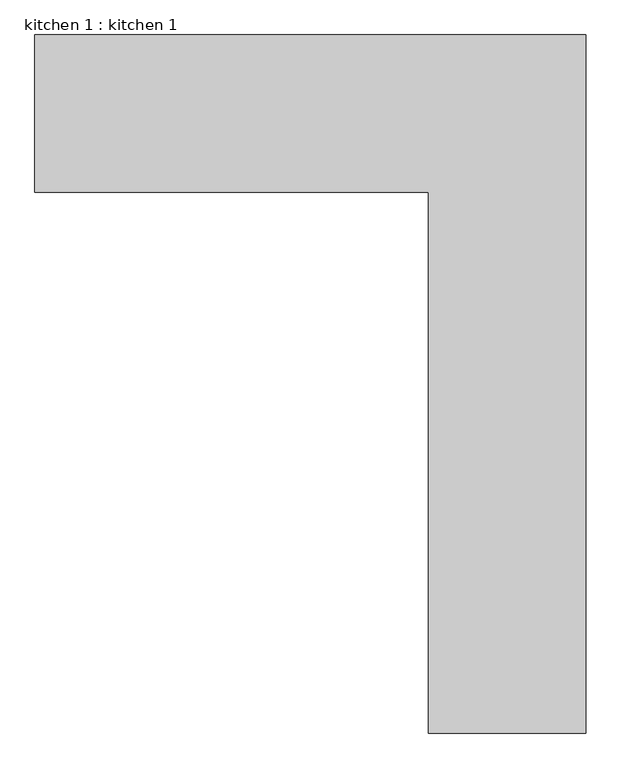
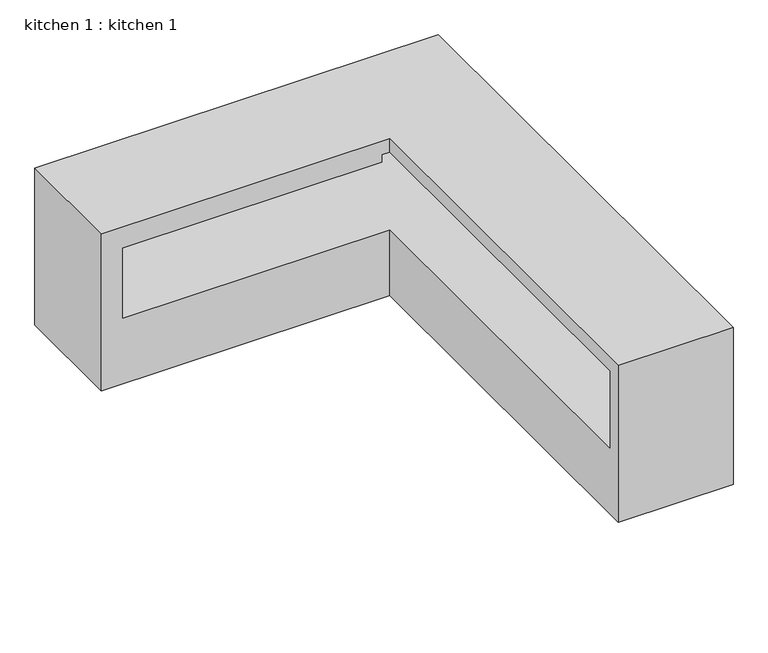
"""IFC4 building model written with IfcOpenShell, lengths in millimetres: proxy geometry, kitchen 1 : kitchen 1."""

from ifc_helpers import new_model, si_unit, origin, place, context, project, spatial, faceted_brep, source, transform, mapped, element, save


def kitchen_1_kitchen_1_5a132608(model_context):
    return source(origin(), model_context, "Body", "Brep", [
        faceted_brep([(655.6395737, 6282.0870892, 609.6), (2246.6994028, 6282.0870892, 609.6), (2246.6994028, 4097.6870892, 609.6), (2881.6994028, 4097.6870892, 609.6), (2881.6994028, 6917.0870892, 609.6), (655.6395737, 6917.0870892, 609.6), (655.6395737, 6282.0870892, -304.8), (655.6395737, 6917.0870892, -304.8), (2881.6994028, 6917.0870892, -304.8), (2881.6994028, 4097.6870892, -304.8), (2246.6994028, 4097.6870892, -304.8), (2246.6994028, 6282.0870892, -304.8), (2246.6994028, 6282.0870892, 76.2), (771.4865087, 6282.0870892, 76.2), (771.4865087, 6282.0870892, 489.2110353), (2202.9571444, 6282.0870892, 489.2110353), (2202.9571444, 6282.0870892, 533.4), (2246.6994028, 6282.0870892, 533.4), (2246.6994028, 4173.8870892, 533.4), (2246.6994028, 4173.8870892, 76.2), (2881.6994028, 6917.0870892, 76.2), (2881.6994028, 4173.8870892, 76.2), (2881.6994028, 4173.8870892, 533.4), (2881.6994028, 6917.0870892, 533.4), (2202.9571444, 6917.0870892, 533.4), (2202.9571444, 6917.0870892, 489.2110353), (771.4865087, 6917.0870892, 489.2110353), (771.4865087, 6917.0870892, 76.2)], [[[0, 1, 2, 3, 4, 5]], [[6, 7, 8, 9, 10, 11]], [[1, 0, 6, 11, 12, 13, 14, 15, 16, 17]], [[2, 1, 17, 18, 19, 12, 11, 10]], [[3, 2, 10, 9]], [[4, 3, 9, 8, 20, 21, 22, 23]], [[5, 4, 23, 24, 25, 26, 27, 20, 8, 7]], [[0, 5, 7, 6]], [[27, 13, 12, 19, 21, 20]], [[13, 27, 26, 14]], [[14, 26, 25, 15]], [[24, 16, 15, 25]], [[16, 24, 23, 22, 18, 17]], [[18, 22, 21, 19]]]),
    ])


if __name__ == "__main__":
    model = new_model("IFC4")
    model_context = context("Model", 3, world=origin())
    ifc_project = project(units=[si_unit("LENGTHUNIT", "METRE", prefix="MILLI")], contexts=[model_context])
    site = spatial("IfcSite", under=ifc_project)
    building = spatial("IfcBuilding", under=site)
    placement = place(None, origin())
    kitchen_1_kitchen_1_shape = kitchen_1_kitchen_1_5a132608(model_context)
    element("IfcBuildingElementProxy", 1, Name="kitchen 1 : kitchen 1", ObjectType="kitchen 1 : kitchen 1", at=placement, inside=building, context=model_context, shape_type="MappedRepresentation", body=[
        mapped(kitchen_1_kitchen_1_shape, transform((0.0, 0.0, 0.0), x_axis=(1.0, 0.0, 0.0), y_axis=(0.0, 1.0, 0.0), z_axis=(0.0, 0.0, 1.0))),
    ])
    save(model, "model.ifc")
